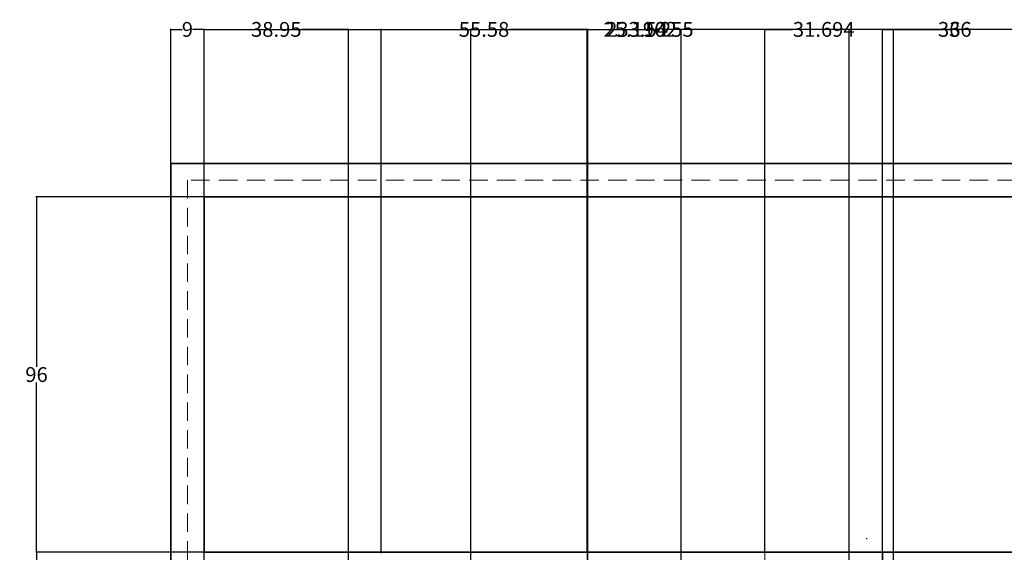
# Model space of a CAD drawing. Units: inches. Extents: x 1291 to 2095, y 532 to 1090.
# Tile 3 of 14: x 1293 to 1559, y 946 to 1090. Entities that reach past the tile are written whole.
import ezdxf

# ---------------------------------------------------------------- set-up
doc = ezdxf.new("R2010")
doc.units = ezdxf.units.IN
doc.header["$MEASUREMENT"] = 0
doc.linetypes.add('HIDDEN', pattern=[0.375, 0.25, -0.125])
for name, color, linetype, lineweight in [('A-ANNO-DIMS', 2, 'Continuous', 18), ('A-GLAZ', 4, 'Continuous', 18), ('A-WALL', 7, 'Continuous', 35), ('A-WALL-HIDN', 8, 'HIDDEN', 13)]:
    doc.layers.add(name, color=color, linetype=linetype, lineweight=lineweight)
doc.styles.get("Standard").update_dxf_attribs({"font": 'arial.ttf'})
doc.dimstyles.get("Standard").update_dxf_attribs({"dimtxt": 4, "dimasz": 0.18, "dimexe": 0.18, "dimexo": 0.0625, "dimgap": 0.09, "dimtad": 0, "dimtih": 1, "dimtoh": 1, "dimdec": 0, "dimrnd": 6, "dimzin": 0, "dimdsep": 46, "dimlunit": 3, "dimtxsty": 'Standard', "dimcen": 0.09, "dimadec": 0, "dimazin": 0, "dimtfac": 1, "dimtdec": 0, "dimtofl": 0, "dimtmove": 0, "dimatfit": 3, "dimfxl": 1, "dimtolj": 1, "dimtzin": 0, "dimarcsym": 0})

# ---------------------------------------------------------------- blocks, each defined once
blk = doc.blocks.new('WIN-48IN')
for points in [[(0, 0), (0, 9), (48, 9), (48, 0)], [(4, 4), (4, 5), (44, 5), (44, 4)]]:
    blk.add_lwpolyline(points, close=True)
blk = doc.blocks.new('*D35')
at = {"layer": 'A-ANNO-DIMS', "color": 0, "lineweight": -2, "transparency": 16777216}
for p, q in [((1343.01, 945.78), (1297.69, 945.78)), ((1297.87, 945.6), (1297.87, 836.88)), ((1297.87, 723.96), (1297.87, 832.68)), ((1343.01, 723.78), (1297.69, 723.78))]:
    blk.add_line(p, q, dxfattribs=at)
at = {"layer": 'A-ANNO-DIMS', "color": 0, "transparency": 16777216}
for points in [[(1297.84, 945.6), (1297.9, 945.6), (1297.87, 945.78)], [(1297.84, 723.96), (1297.9, 723.96), (1297.87, 723.78)]]:
    blk.add_solid(points, dxfattribs=at)
at = {"layer": 'Defpoints', "color": 0, "transparency": 16777216}
for p in [(1297.87, 945.78), (1343.07, 945.78), (1343.07, 723.78)]:
    blk.add_point(p, dxfattribs=at)
at = {"layer": 'A-ANNO-DIMS', "color": 0, "transparency": 16777216, "insert": (1297.87, 834.78), "char_height": 4, "attachment_point": 5}
blk.add_mtext('\\A1;222', dxfattribs=at)
blk = doc.blocks.new('*D36')
at = {"layer": 'A-ANNO-DIMS', "color": 0, "lineweight": -2, "transparency": 16777216}
for p, q in [((1343.01, 1041.78), (1297.69, 1041.78)), ((1297.87, 1041.6), (1297.87, 995.91)), ((1297.87, 945.96), (1297.87, 991.65)), ((1343.01, 945.78), (1297.69, 945.78))]:
    blk.add_line(p, q, dxfattribs=at)
at = {"layer": 'A-ANNO-DIMS', "color": 0, "transparency": 16777216}
for points in [[(1297.84, 1041.6), (1297.9, 1041.6), (1297.87, 1041.78)], [(1297.84, 945.96), (1297.9, 945.96), (1297.87, 945.78)]]:
    blk.add_solid(points, dxfattribs=at)
at = {"layer": 'Defpoints', "color": 0, "transparency": 16777216}
for p in [(1297.87, 1041.78), (1343.07, 1041.78), (1343.07, 945.78)]:
    blk.add_point(p, dxfattribs=at)
at = {"layer": 'A-ANNO-DIMS', "color": 0, "transparency": 16777216, "insert": (1297.87, 993.78), "char_height": 4, "attachment_point": 5}
blk.add_mtext('\\A1;96', dxfattribs=at)
blk = doc.blocks.new('*D37')
at = {"layer": 'A-ANNO-DIMS', "color": 0, "lineweight": -2, "transparency": 16777216}
for p, q in [((1334.07, 1050.84), (1334.07, 1087.16)), ((1334.25, 1086.98), (1337.17, 1086.98)), ((1342.89, 1086.98), (1339.98, 1086.98)), ((1343.07, 1041.84), (1343.07, 1087.16))]:
    blk.add_line(p, q, dxfattribs=at)
at = {"layer": 'A-ANNO-DIMS', "color": 0, "transparency": 16777216}
for points in [[(1334.25, 1087.01), (1334.25, 1086.95), (1334.07, 1086.98)], [(1342.89, 1087.01), (1342.89, 1086.95), (1343.07, 1086.98)]]:
    blk.add_solid(points, dxfattribs=at)
at = {"layer": 'Defpoints', "color": 0, "transparency": 16777216}
for p in [(1343.07, 1086.98), (1334.07, 1050.78), (1343.07, 1041.78)]:
    blk.add_point(p, dxfattribs=at)
at = {"layer": 'A-ANNO-DIMS', "color": 0, "transparency": 16777216, "insert": (1338.57, 1086.98), "char_height": 4, "attachment_point": 5}
blk.add_mtext('\\A1;9', dxfattribs=at)
blk = doc.blocks.new('*D38')
at = {"layer": 'A-ANNO-DIMS', "color": 0, "lineweight": -2, "transparency": 16777216}
for p, q in [((1343.07, 1041.84), (1343.07, 1087.16)), ((1343.25, 1086.98), (1466.02, 1086.98)), ((1597.89, 1086.98), (1475.13, 1086.98)), ((1598.07, 1041.84), (1598.07, 1087.16))]:
    blk.add_line(p, q, dxfattribs=at)
at = {"layer": 'A-ANNO-DIMS', "color": 0, "transparency": 16777216}
for points in [[(1343.25, 1087.01), (1343.25, 1086.95), (1343.07, 1086.98)], [(1597.89, 1087.01), (1597.89, 1086.95), (1598.07, 1086.98)]]:
    blk.add_solid(points, dxfattribs=at)
at = {"layer": 'Defpoints', "color": 0, "transparency": 16777216}
for p in [(1598.07, 1086.98), (1343.07, 1041.78), (1598.07, 1041.78)]:
    blk.add_point(p, dxfattribs=at)
at = {"layer": 'A-ANNO-DIMS', "color": 0, "transparency": 16777216, "insert": (1470.57, 1086.98), "char_height": 4, "attachment_point": 5}
blk.add_mtext('\\A1;255', dxfattribs=at)
blk = doc.blocks.new('*D44')
at = {"layer": 'A-ANNO-DIMS', "color": 0, "lineweight": -2, "transparency": 16777216}
for p, q in [((1343.07, 579.84), (1343.07, 1087.16)), ((1343.25, 1086.98), (1451.42, 1086.98)), ((1576.43, 1086.98), (1468.26, 1086.98)), ((1576.61, 579.84), (1576.61, 1087.16))]:
    blk.add_line(p, q, dxfattribs=at)
at = {"layer": 'A-ANNO-DIMS', "color": 0, "transparency": 16777216}
for points in [[(1343.25, 1087.01), (1343.25, 1086.95), (1343.07, 1086.98)], [(1576.43, 1087.01), (1576.43, 1086.95), (1576.61, 1086.98)]]:
    blk.add_solid(points, dxfattribs=at)
at = {"layer": 'Defpoints', "color": 0, "transparency": 16777216}
for p in [(1576.61, 1086.98), (1343.07, 579.78), (1576.61, 579.78)]:
    blk.add_point(p, dxfattribs=at)
at = {"layer": 'A-ANNO-DIMS', "color": 0, "transparency": 16777216, "insert": (1459.84, 1086.98), "char_height": 4, "attachment_point": 5}
blk.add_mtext('\\A1;233.54', dxfattribs=at)
blk = doc.blocks.new('*D54')
at = {"layer": 'A-ANNO-DIMS', "color": 0, "lineweight": -2, "transparency": 16777216}
for p, q in [((1415.07, 861.91), (1415.07, 1087.16)), ((1415.25, 1086.98), (1461.77, 1086.98)), ((1516.89, 1086.98), (1470.37, 1086.98)), ((1517.07, 861.91), (1517.07, 1087.16))]:
    blk.add_line(p, q, dxfattribs=at)
at = {"layer": 'A-ANNO-DIMS', "color": 0, "transparency": 16777216}
for points in [[(1415.25, 1087.01), (1415.25, 1086.95), (1415.07, 1086.98)], [(1516.89, 1087.01), (1516.89, 1086.95), (1517.07, 1086.98)]]:
    blk.add_solid(points, dxfattribs=at)
at = {"layer": 'Defpoints', "color": 0, "transparency": 16777216}
for p in [(1517.07, 1086.98), (1415.07, 861.85), (1517.07, 861.85)]:
    blk.add_point(p, dxfattribs=at)
at = {"layer": 'A-ANNO-DIMS', "color": 0, "transparency": 16777216, "insert": (1466.07, 1086.98), "char_height": 4, "attachment_point": 5}
blk.add_mtext('\\A1;102', dxfattribs=at)
blk = doc.blocks.new('*D61')
at = {"layer": 'A-ANNO-DIMS', "color": 0, "lineweight": -2, "transparency": 16777216}
for p, q in [((1343.07, 732.84), (1343.07, 1087.16)), ((1343.25, 1086.98), (1355.7, 1086.98)), ((1381.84, 1086.98), (1369.4, 1086.98)), ((1382.02, 732.91), (1382.02, 1087.16))]:
    blk.add_line(p, q, dxfattribs=at)
at = {"layer": 'A-ANNO-DIMS', "color": 0, "transparency": 16777216}
for points in [[(1343.25, 1087.01), (1343.25, 1086.95), (1343.07, 1086.98)], [(1381.84, 1087.01), (1381.84, 1086.95), (1382.02, 1086.98)]]:
    blk.add_solid(points, dxfattribs=at)
at = {"layer": 'Defpoints', "color": 0, "transparency": 16777216}
for p in [(1382.02, 1086.98), (1343.07, 732.78), (1382.02, 732.85)]:
    blk.add_point(p, dxfattribs=at)
at = {"layer": 'A-ANNO-DIMS', "color": 0, "transparency": 16777216, "insert": (1362.55, 1086.98), "char_height": 4, "attachment_point": 5}
blk.add_mtext('\\A1;38.95', dxfattribs=at)
blk = doc.blocks.new('*D63')
at = {"layer": 'A-ANNO-DIMS', "color": 0, "lineweight": -2, "transparency": 16777216}
for p, q in [((1529.07, 723.84), (1529.07, 1087.16)), ((1529.25, 1086.98), (1544.12, 1086.98)), ((1564.89, 1086.98), (1550.03, 1086.98)), ((1565.07, 723.84), (1565.07, 1087.16))]:
    blk.add_line(p, q, dxfattribs=at)
at = {"layer": 'A-ANNO-DIMS', "color": 0, "transparency": 16777216}
for points in [[(1529.25, 1087.01), (1529.25, 1086.95), (1529.07, 1086.98)], [(1564.89, 1087.01), (1564.89, 1086.95), (1565.07, 1086.98)]]:
    blk.add_solid(points, dxfattribs=at)
at = {"layer": 'Defpoints', "color": 0, "transparency": 16777216}
for p in [(1565.07, 1086.98), (1529.07, 723.78), (1565.07, 723.78)]:
    blk.add_point(p, dxfattribs=at)
at = {"layer": 'A-ANNO-DIMS', "color": 0, "transparency": 16777216, "insert": (1547.07, 1086.98), "char_height": 4, "attachment_point": 5}
blk.add_mtext('\\A1;36', dxfattribs=at)
blk = doc.blocks.new('*D69')
at = {"layer": 'A-ANNO-DIMS', "color": 0, "lineweight": -2, "transparency": 16777216}
for p, q in [((1390.8, 945.53), (1390.8, 1087.16)), ((1390.98, 1086.98), (1411.75, 1086.98)), ((1446.2, 1086.98), (1425.43, 1086.98)), ((1446.38, 945.99), (1446.38, 1087.16))]:
    blk.add_line(p, q, dxfattribs=at)
at = {"layer": 'A-ANNO-DIMS', "color": 0, "transparency": 16777216}
for points in [[(1390.98, 1087.01), (1390.98, 1086.95), (1390.8, 1086.98)], [(1446.2, 1087.01), (1446.2, 1086.95), (1446.38, 1086.98)]]:
    blk.add_solid(points, dxfattribs=at)
at = {"layer": 'Defpoints', "color": 0, "transparency": 16777216}
for p in [(1446.38, 1086.98), (1446.38, 945.92), (1390.8, 945.47)]:
    blk.add_point(p, dxfattribs=at)
at = {"layer": 'A-ANNO-DIMS', "color": 0, "transparency": 16777216, "insert": (1418.59, 1086.98), "char_height": 4, "attachment_point": 5}
blk.add_mtext('\\A1;55.58', dxfattribs=at)
blk = doc.blocks.new('*D70')
at = {"layer": 'A-ANNO-DIMS', "color": 0, "lineweight": -2, "transparency": 16777216}
for p, q in [((1494.38, 945.99), (1494.38, 1087.16)), ((1494.56, 1086.98), (1501.84, 1086.98)), ((1525.89, 1086.98), (1518.61, 1086.98)), ((1526.07, 945.84), (1526.07, 1087.16))]:
    blk.add_line(p, q, dxfattribs=at)
at = {"layer": 'A-ANNO-DIMS', "color": 0, "transparency": 16777216}
for points in [[(1494.56, 1087.01), (1494.56, 1086.95), (1494.38, 1086.98)], [(1525.89, 1087.01), (1525.89, 1086.95), (1526.07, 1086.98)]]:
    blk.add_solid(points, dxfattribs=at)
at = {"layer": 'Defpoints', "color": 0, "transparency": 16777216}
for p in [(1526.07, 1086.98), (1494.38, 945.92), (1526.07, 945.78)]:
    blk.add_point(p, dxfattribs=at)
at = {"layer": 'A-ANNO-DIMS', "color": 0, "transparency": 16777216, "insert": (1510.23, 1086.98), "char_height": 4, "attachment_point": 5}
blk.add_mtext('\\A1;31.694', dxfattribs=at)
blk = doc.blocks.new('*D71')
at = {"layer": 'A-ANNO-DIMS', "color": 0, "lineweight": -2, "transparency": 16777216}
for p, q in [((1526.07, 945.84), (1526.07, 1087.16)), ((1526.25, 1086.98), (1541.12, 1086.98)), ((1561.89, 1086.98), (1547.03, 1086.98)), ((1562.07, 945.84), (1562.07, 1087.16))]:
    blk.add_line(p, q, dxfattribs=at)
at = {"layer": 'A-ANNO-DIMS', "color": 0, "transparency": 16777216}
for points in [[(1526.25, 1087.01), (1526.25, 1086.95), (1526.07, 1086.98)], [(1561.89, 1087.01), (1561.89, 1086.95), (1562.07, 1086.98)]]:
    blk.add_solid(points, dxfattribs=at)
at = {"layer": 'Defpoints', "color": 0, "transparency": 16777216}
for p in [(1562.07, 1086.98), (1526.07, 945.78), (1562.07, 945.78)]:
    blk.add_point(p, dxfattribs=at)
at = {"layer": 'A-ANNO-DIMS', "color": 0, "transparency": 16777216, "insert": (1544.07, 1086.98), "char_height": 4, "attachment_point": 5}
blk.add_mtext('\\A1;36', dxfattribs=at)
blk = doc.blocks.new('*D82')
at = {"layer": 'A-ANNO-DIMS', "color": 0, "lineweight": -2, "transparency": 16777216}
for p, q in [((1446.55, 823.54), (1446.55, 1087.16)), ((1446.73, 1086.98), (1450.72, 1086.98)), ((1471.56, 1086.98), (1467.57, 1086.98)), ((1471.74, 823.54), (1471.74, 1087.16))]:
    blk.add_line(p, q, dxfattribs=at)
at = {"layer": 'A-ANNO-DIMS', "color": 0, "transparency": 16777216}
for points in [[(1446.73, 1087.01), (1446.73, 1086.95), (1446.55, 1086.98)], [(1471.56, 1087.01), (1471.56, 1086.95), (1471.74, 1086.98)]]:
    blk.add_solid(points, dxfattribs=at)
at = {"layer": 'Defpoints', "color": 0, "transparency": 16777216}
for p in [(1471.74, 1086.98), (1446.55, 823.47), (1471.74, 823.47)]:
    blk.add_point(p, dxfattribs=at)
at = {"layer": 'A-ANNO-DIMS', "color": 0, "transparency": 16777216, "insert": (1459.15, 1086.98), "char_height": 4, "attachment_point": 5}
blk.add_mtext('\\A1;25.196', dxfattribs=at)
blk = doc.blocks.new('*D90')
at = {"layer": 'A-ANNO-DIMS', "color": 0, "lineweight": -2, "transparency": 16777216}
for p, q in [((1521.76, 949.52), (1521.94, 949.52)), ((1521.85, 949.43), (1521.85, 949.61)), ((1533.8, 886), (1529.35, 909.64)), ((1533.98, 886), (1533.8, 886))]:
    blk.add_line(p, q, dxfattribs=at)
at = {"layer": 'A-ANNO-DIMS', "color": 0, "transparency": 16777216}
blk.add_solid([(1529.38, 909.65), (1529.32, 909.63), (1529.32, 909.82)], dxfattribs=at)
at = {"layer": 'Defpoints', "color": 0, "transparency": 16777216}
for p in [(1521.85, 949.52), (1529.32, 909.82)]:
    blk.add_point(p, dxfattribs=at)
at = {"layer": 'A-ANNO-DIMS', "color": 0, "transparency": 16777216, "insert": (1541.17, 886), "char_height": 4, "attachment_point": 5}
blk.add_mtext('\\A1;R40.4', dxfattribs=at)

msp = doc.modelspace()

# ---------------------------------------------------------------- linework, layer by layer
at = {"layer": 'A-WALL'}
for p, q in [((2054.0735, 1050.7804), (1334.0735, 1050.7804)), ((1334.0735, 1050.7804), (1334.0735, 570.7804)), ((1343.0735, 1041.7804), (1343.0735, 945.7804)), ((1694.0735, 1041.7804), (1343.0735, 1041.7804)), ((1526.0735, 945.7804), (1343.0735, 945.7804)), ((1526.0735, 936.7804), (1526.0735, 945.7804)), ((1694.0735, 945.7804), (1526.0735, 945.7804))]:
    msp.add_line(p, q, dxfattribs=at)
at = {"layer": 'A-WALL-HIDN', "ltscale": 20}
for p, q in [((2049.5735, 1046.2804), (1338.5735, 1046.2804)), ((1338.5735, 1046.2804), (1338.5735, 570.7804))]:
    msp.add_line(p, q, dxfattribs=at)

# ---------------------------------------------------------------- block references
at = {"layer": 'A-GLAZ'}
msp.add_blockref('WIN-48IN', (1446.3793, 936.9233), dxfattribs=at)

# ---------------------------------------------------------------- dimensions: what is measured, and where the dimension line sits
at = {"layer": 'A-ANNO-DIMS'}
for base, p1, p2, override, picture, middle in [((1343.0735, 1086.9804), (1334.0735, 1050.7804), (1343.0735, 1041.7804), {"dimdec": 0, "dimlfac": 1, "dimrnd": 0, "dimzin": 0, "dimdsep": 46, "dimlunit": 2}, '*D37', (1338.5735, 1086.9804)), ((1598.0735, 1086.9804), (1343.0735, 1041.7804), (1598.0735, 1041.7804), {"dimdec": 0, "dimlfac": 1, "dimrnd": 0, "dimzin": 0, "dimdsep": 46, "dimlunit": 2}, '*D38', (1470.5735, 1086.9804)), ((1576.6107, 1086.9804), (1343.0735, 579.7804), (1576.6107, 579.7804), {"dimdec": 2, "dimlfac": 1, "dimrnd": 0, "dimzin": 0, "dimdsep": 46, "dimlunit": 2}, '*D44', (1459.8421, 1086.9804)), ((1382.0234, 1086.9804), (1343.0735, 732.7804), (1382.0234, 732.8453), {"dimdec": 2, "dimlfac": 1, "dimrnd": 0, "dimzin": 0, "dimdsep": 46, "dimlunit": 2}, '*D61', (1362.5485, 1086.9804)), ((1446.3797, 1086.9804), (1390.7986, 945.4707), (1446.3797, 945.9238), {"dimdec": 2, "dimlfac": 1, "dimrnd": 0, "dimzin": 0, "dimdsep": 46, "dimlunit": 2}, '*D69', (1418.5892, 1086.9804)), ((1517.0658, 1086.9804), (1415.0735, 861.8516), (1517.0658, 861.8516), {"dimdec": 0, "dimlfac": 1, "dimrnd": 0, "dimzin": 0, "dimdsep": 46, "dimlunit": 2}, '*D54', (1466.0697, 1086.9804)), ((1471.7436, 1086.9804), (1446.5476, 823.4737), (1471.7436, 823.4737), {"dimdec": 3, "dimlfac": 1, "dimrnd": 0, "dimzin": 0, "dimdsep": 46, "dimlunit": 2}, '*D82', (1459.1456, 1086.9804)), ((1526.0735, 1086.9804), (1494.3797, 945.9238), (1526.0735, 945.7804), {"dimdec": 3, "dimlfac": 1, "dimrnd": 0, "dimzin": 0, "dimdsep": 46, "dimlunit": 2}, '*D70', (1510.2266, 1086.9804)), ((1562.0735, 1086.9804), (1526.0735, 945.7804), (1562.0735, 945.7804), {"dimdec": 0, "dimlfac": 1, "dimrnd": 0, "dimzin": 0, "dimdsep": 46, "dimlunit": 2}, '*D71', (1544.0735, 1086.9804)), ((1565.0735, 1086.9804), (1529.0735, 723.7804), (1565.0735, 723.7804), {"dimdec": 0, "dimlfac": 1, "dimrnd": 0, "dimzin": 0, "dimdsep": 46, "dimlunit": 2}, '*D63', (1547.0735, 1086.9804))]:
    dim = msp.add_linear_dim(base=base, p1=p1, p2=p2, dimstyle='Standard', override=override, dxfattribs=at)
    dim.commit()
    dim.dimension.update_dxf_attribs({"geometry": picture, "text_midpoint": middle})
for base, p1, p2, picture, middle in [((1297.8735, 1041.7804), (1343.0735, 945.7804), (1343.0735, 1041.7804), '*D36', (1297.8735, 993.7804)), ((1297.8735, 945.7804), (1343.0735, 723.7804), (1343.0735, 945.7804), '*D35', (1297.8735, 834.7804))]:
    dim = msp.add_linear_dim(base=base, p1=p1, p2=p2, angle=90, dimstyle='Standard', override={"dimdec": 0, "dimlfac": 1, "dimrnd": 0, "dimzin": 0, "dimdsep": 46, "dimlunit": 2}, dxfattribs=at)
    dim.commit()
    dim.dimension.update_dxf_attribs({"geometry": picture, "text_midpoint": middle})
dim = msp.add_radius_dim(center=(1521.8491, 949.5186), mpoint=(1529.3156, 909.8169), dimstyle='Standard', override={"dimdec": 1, "dimlfac": 1, "dimrnd": 0, "dimzin": 0, "dimdsep": 46, "dimlunit": 2}, dxfattribs=at)
dim.commit()
dim.dimension.update_dxf_attribs({"geometry": '*D90', "text_midpoint": (1541.1665, 885.9958), "dimtype": 164})

doc.saveas('drawing.dxf')
